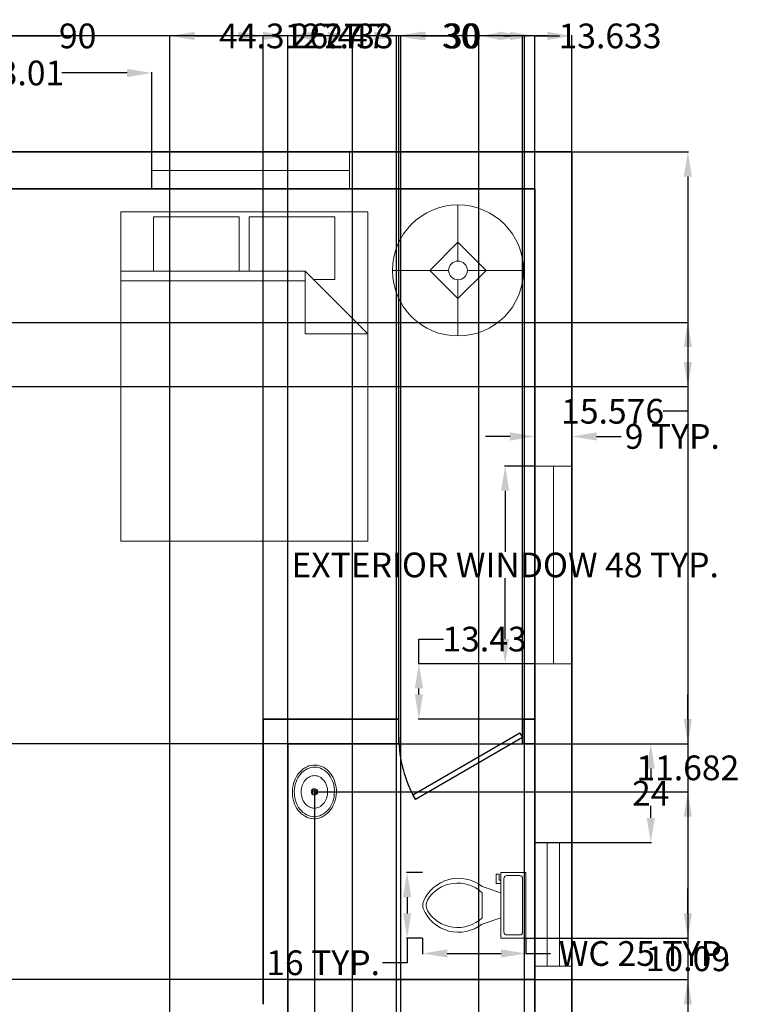
# Model space of a CAD drawing. Units: inches. Extents: x 351 to 774, y 111 to 703.
# Tile 6 of 6: x 599 to 774, y 464 to 703. Entities that reach past the tile are written whole.
import ezdxf

# ---------------------------------------------------------------- set-up
doc = ezdxf.new("R2010")
doc.units = ezdxf.units.IN
doc.header["$MEASUREMENT"] = 0
for name, color, linetype, lineweight in [('A-ANNO-DIMS', 2, 'Continuous', 18), ('A-DOOR', 3, 'Continuous', 25), ('A-FLOR-FIXT', 9, 'Continuous', 18), ('A-FURN', 8, 'Continuous', 18), ('A-GLAZ', 4, 'Continuous', 18), ('A-WALL', 7, 'Continuous', 35)]:
    doc.layers.add(name, color=color, linetype=linetype, lineweight=lineweight)
doc.styles.get("Standard").update_dxf_attribs({"font": 'arial.ttf'})
doc.dimstyles.get("Standard").update_dxf_attribs({"dimtxt": 6, "dimasz": 6, "dimexe": 0.18, "dimexo": 0.0625, "dimgap": 0.09, "dimtad": 0, "dimtih": 1, "dimtoh": 1, "dimdec": 0, "dimzin": 0, "dimdsep": 46, "dimlunit": 3, "dimtxsty": 'Standard', "dimcen": 0.09, "dimadec": 0, "dimazin": 0, "dimtfac": 1, "dimtdec": 0, "dimtofl": 0, "dimtmove": 0, "dimatfit": 3, "dimfxl": 1, "dimtolj": 1, "dimtzin": 0, "dimarcsym": 0})

# ---------------------------------------------------------------- blocks, each defined once
blk = doc.blocks.new('*U4')
for p, q in [((-40, 0), (-40, 6)), ((0, 0), (0, 6))]:
    blk.add_line(p, q)
blk.add_lwpolyline([(0, 0), (-34.64, -20), (-35.52, -18.48), (-0.88, 1.52)], close=True)
blk.add_arc((0, 0), 40, 180, 210)
blk = doc.blocks.new('Bed - Queen')
for p, q in [((0, -80.00003), (0, 0)), ((0, 0), (59.99999, 0)), ((59.99999, 0), (59.99999, -80.00003)), ((7.99999, -1.2), (28.79998, -1.2)), ((7.99999, -14.4), (7.99999, -1.2)), ((28.79998, -1.2), (28.79998, -14.4)), ((31.19999, -1.2), (51.99999, -1.2)), ((31.19999, -14.4), (31.19999, -1.2)), ((51.99999, -1.2), (51.99999, -16.4)), ((0, -14.4), (44.8, -14.4)), ((59.99999, -29.6), (44.8, -14.4)), ((44.8, -14.4), (44.8, -29.6)), ((51.99999, -16.4), (46.79936, -16.4)), ((44.8, -16.8), (0, -16.8)), ((44.8, -29.6), (59.99999, -29.6)), ((59.99999, -80.00003), (0, -80.00003))]:
    blk.add_line(p, q)
blk = doc.blocks.new('Lamp - Table')
for p, q in [((0, 7), (0, 1)), ((0, 3), (-3, 0)), ((3, 0), (0, 3)), ((-1, 0), (-7, 0)), ((-3, 0), (0, -3)), ((0, -3), (3, 0)), ((1, 0), (7, 0)), ((0, -1), (0, -7))]:
    blk.add_line(p, q)
for radius in [7, 1]:
    blk.add_circle((0, 0), radius)
blk = doc.blocks.new('Toilet - top')
for p, q in [((9.5, -6), (9.5, -2)), ((-10, -8.5), (-8, -8.5)), ((-10, -9.5), (-10, -8.5)), ((-8, -8.5), (-8, -8)), ((-7, -8), (-7, -9.5)), ((-4, -8), (-6, -14)), ((4, -8), (6, -14)), ((-7, -9.5), (-10, -9.5)), ((4, -14), (-4, -14))]:
    blk.add_line(p, q)
blk.add_lwpolyline([(10.5, -8), (10.5, 0), (-10.5, 0), (-10.5, -8)], close=True)
for points in [[(-9.5, -2), (-9.5, -6)], [(8.5, -1), (-8.5, -1)], [(-8.5, -7), (8.5, -7)]]:
    blk.add_lwpolyline(points)
for centre, radius, start, end in [((-8.62, -1.88), 0.884, 81.8699, 188.1301), ((8.62, -1.88), 0.884, 351.8699, 98.1301), ((-8.62, -6.12), 0.884, 171.8699, 278.1301), ((8.62, -6.12), 0.884, 261.8699, 8.1301), ((3.52, -21.58), 12.17, 141.4691, 247.9714), ((4.2, -21.82), 11.33, 136.3677, 238.9468), ((-3.52, -21.58), 12.17, 292.0284, 38.5307), ((-4.2, -21.82), 11.33, 301.053, 43.6321), ((0, -27.88), 4, 245.7318, 294.2682), ((0, -29), 4, 254.8605, 285.1395)]:
    blk.add_arc(centre, radius, start, end)
blk = doc.blocks.new('Sink - Oval top')
for p, q in [((-1, 0), (1, 0)), ((0, 1), (0, -1))]:
    blk.add_line(p, q)
for points in [[(-12.23, 0.39, 0.117634), (-11.46, -3.36, 0.104469), (-8.88, -6.8, 0.090016), (-5.08, -9.07, 0.08192), (-0.32, -10.02, 0.08192), (4.49, -9.38, 0.090016), (8.42, -7.36, 0.104469), (11.22, -4.09, 0.117634), (12.23, -0.39, 0.117634), (11.46, 3.36, 0.104469), (8.88, 6.8, 0.090016), (5.08, 9.07, 0.08192), (0.32, 10.02, 0.08192), (-4.49, 9.38, 0.090016), (-8.42, 7.36, 0.104469), (-11.22, 4.09, 0.117634)], [(-11.29, 0.16, 0.118622), (-10.52, -3.25, 0.104678), (-8.07, -6.36, 0.089562), (-4.54, -8.37, 0.081185), (-0.13, -9.15, 0.081185), (4.3, -8.49, 0.089562), (7.89, -6.58, 0.104678), (10.42, -3.55, 0.118622), (11.29, -0.16, 0.118622), (10.52, 3.25, 0.104678), (8.07, 6.36, 0.089562), (4.54, 8.37, 0.081185), (0.13, 9.15, 0.081185), (-4.3, 8.49, 0.089562), (-7.89, 6.58, 0.104678), (-10.42, 3.55, 0.118622)], [(-7.42, 0.08, 0.118283), (-6.91, -2.17, 0.104607), (-5.29, -4.21, 0.089718), (-2.97, -5.53, 0.081436), (-0.07, -6.04, 0.081436), (2.84, -5.59, 0.089718), (5.2, -4.33, 0.104607), (6.86, -2.32, 0.118283), (7.42, -0.08, 0.118283), (6.91, 2.17, 0.104607), (5.29, 4.21, 0.089718), (2.97, 5.53, 0.081436), (0.07, 6.04, 0.081436), (-2.84, 5.59, 0.089718), (-5.2, 4.33, 0.104607), (-6.86, 2.32, 0.118283)]]:
    blk.add_lwpolyline(points, format="xyb", close=True)
for radius in [1.5, 1]:
    blk.add_circle((0, 0), radius)
blk = doc.blocks.new('WIN-48IN-9IN-WALL')
blk.add_line((4.5, 48), (4.5, 0))
blk.add_lwpolyline([(0, 0), (9, 0), (9, 48), (0, 48)], close=True)
blk = doc.blocks.new('WIN-BATH-30IN-9IN-WALL')
for p, q in [((0, 0), (0, 9)), ((0, 9), (30, 9)), ((30, 9), (30, 0)), ((0, 6), (30, 6)), ((30, 3), (0, 3)), ((30, 0), (0, 0))]:
    blk.add_line(p, q)
blk = doc.blocks.new('*D24')
at = {"layer": 'A-ANNO-DIMS', "color": 0, "lineweight": -2, "transparency": 16777216}
for p, q in [((723.98, 594.93), (716.66, 594.93)), ((716.84, 588.93), (716.84, 574.13)), ((716.84, 552.93), (716.84, 567.74)), ((723.98, 546.93), (716.66, 546.93))]:
    blk.add_line(p, q, dxfattribs=at)
at = {"layer": 'A-ANNO-DIMS', "color": 0, "transparency": 16777216}
for points in [[(715.84, 588.93), (717.84, 588.93), (716.84, 594.93)], [(715.84, 552.93), (717.84, 552.93), (716.84, 546.93)]]:
    blk.add_solid(points, dxfattribs=at)
at = {"layer": 'Defpoints', "color": 0, "transparency": 16777216}
for p in [(716.84, 594.93), (724.04, 594.93), (724.04, 546.93)]:
    blk.add_point(p, dxfattribs=at)
at = {"layer": 'A-ANNO-DIMS', "color": 0, "transparency": 16777216, "insert": (716.84, 570.93), "char_height": 6, "attachment_point": 5}
blk.add_mtext('\\A1;EXTERIOR WINDOW 48 TYP.', dxfattribs=at)
blk = doc.blocks.new('*D25')
at = {"layer": 'A-ANNO-DIMS', "color": 0, "lineweight": -2, "transparency": 16777216}
for p, q in [((718.04, 602.13), (712.04, 602.13)), ((724.04, 594.99), (724.04, 602.31)), ((733.04, 594.99), (733.04, 602.31)), ((739.04, 602.13), (745.04, 602.13))]:
    blk.add_line(p, q, dxfattribs=at)
at = {"layer": 'A-ANNO-DIMS', "color": 0, "transparency": 16777216}
for points in [[(718.04, 603.13), (718.04, 601.13), (724.04, 602.13)], [(739.04, 603.13), (739.04, 601.13), (733.04, 602.13)]]:
    blk.add_solid(points, dxfattribs=at)
at = {"layer": 'Defpoints', "color": 0, "transparency": 16777216}
for p in [(733.04, 602.13), (724.04, 594.93), (733.04, 594.93)]:
    blk.add_point(p, dxfattribs=at)
at = {"layer": 'A-ANNO-DIMS', "color": 0, "transparency": 16777216, "insert": (757.41, 602.13), "char_height": 6, "attachment_point": 5}
blk.add_mtext('\\A1;9 TYP.', dxfattribs=at)
blk = doc.blocks.new('*D32')
at = {"layer": 'A-ANNO-DIMS', "color": 0, "lineweight": -2, "transparency": 16777216}
for p, q in [((696.79, 480.27), (696.79, 476.4)), ((721.84, 480.27), (721.84, 476.4)), ((702.79, 476.58), (715.84, 476.58)), ((721.84, 476.58), (727.84, 476.58))]:
    blk.add_line(p, q, dxfattribs=at)
at = {"layer": 'A-ANNO-DIMS', "color": 0, "transparency": 16777216}
for points in [[(702.79, 477.58), (702.79, 475.58), (696.79, 476.58)], [(715.84, 477.58), (715.84, 475.58), (721.84, 476.58)]]:
    blk.add_solid(points, dxfattribs=at)
at = {"layer": 'Defpoints', "color": 0, "transparency": 16777216}
for p in [(696.79, 480.33), (721.84, 480.33), (721.84, 476.58)]:
    blk.add_point(p, dxfattribs=at)
at = {"layer": 'A-ANNO-DIMS', "color": 0, "transparency": 16777216, "insert": (750.8, 476.58), "char_height": 6, "attachment_point": 5}
blk.add_mtext('\\A1;WC 25 TYP.', dxfattribs=at)
blk = doc.blocks.new('*D33')
at = {"layer": 'A-ANNO-DIMS', "color": 0, "lineweight": -2, "transparency": 16777216}
for p, q in [((696.73, 496.24), (692.86, 496.24)), ((693.04, 490.24), (693.04, 486.33)), ((696.73, 480.33), (692.86, 480.33)), ((693.04, 480.33), (693.04, 474.33)), ((693.04, 474.33), (687.04, 474.33))]:
    blk.add_line(p, q, dxfattribs=at)
at = {"layer": 'A-ANNO-DIMS', "color": 0, "transparency": 16777216}
for points in [[(692.04, 490.24), (694.04, 490.24), (693.04, 496.24)], [(692.04, 486.33), (694.04, 486.33), (693.04, 480.33)]]:
    blk.add_solid(points, dxfattribs=at)
at = {"layer": 'Defpoints', "color": 0, "transparency": 16777216}
for p in [(696.79, 496.24), (693.04, 480.33), (696.79, 480.33)]:
    blk.add_point(p, dxfattribs=at)
at = {"layer": 'A-ANNO-DIMS', "color": 0, "transparency": 16777216, "insert": (672.63, 474.33), "char_height": 6, "attachment_point": 5}
blk.add_mtext('\\A1;16 TYP.', dxfattribs=at)
blk = doc.blocks.new('*D46')
at = {"layer": 'A-ANNO-DIMS', "color": 0, "lineweight": -2, "transparency": 16777216}
for p, q in [((421.04, 671.3), (421.04, 699.57)), ((427.04, 699.39), (570.36, 699.39)), ((727.04, 699.39), (583.73, 699.39)), ((733.04, 671.3), (733.04, 699.57))]:
    blk.add_line(p, q, dxfattribs=at)
at = {"layer": 'A-ANNO-DIMS', "color": 0, "transparency": 16777216}
for points in [[(427.04, 700.39), (427.04, 698.39), (421.04, 699.39)], [(727.04, 700.39), (727.04, 698.39), (733.04, 699.39)]]:
    blk.add_solid(points, dxfattribs=at)
at = {"layer": 'Defpoints', "color": 0, "transparency": 16777216}
for p in [(733.04, 699.39), (421.04, 671.24), (733.04, 671.24)]:
    blk.add_point(p, dxfattribs=at)
at = {"layer": 'A-ANNO-DIMS', "color": 0, "transparency": 16777216, "insert": (577.04, 699.39), "char_height": 6, "attachment_point": 5}
blk.add_mtext('\\A1;312', dxfattribs=at)
blk = doc.blocks.new('*D47')
at = {"layer": 'A-ANNO-DIMS', "color": 0, "lineweight": -2, "transparency": 16777216}
for p, q in [((733.11, 671.24), (761.37, 671.24)), ((761.19, 665.24), (761.19, 410.4)), ((761.19, 149.24), (761.19, 404.09)), ((733.11, 143.24), (761.37, 143.24))]:
    blk.add_line(p, q, dxfattribs=at)
at = {"layer": 'A-ANNO-DIMS', "color": 0, "transparency": 16777216}
for points in [[(760.19, 665.24), (762.19, 665.24), (761.19, 671.24)], [(760.19, 149.24), (762.19, 149.24), (761.19, 143.24)]]:
    blk.add_solid(points, dxfattribs=at)
at = {"layer": 'Defpoints', "color": 0, "transparency": 16777216}
for p in [(733.04, 671.24), (761.19, 671.24), (733.04, 143.24)]:
    blk.add_point(p, dxfattribs=at)
at = {"layer": 'A-ANNO-DIMS', "color": 0, "transparency": 16777216, "insert": (761.19, 407.24), "char_height": 6, "attachment_point": 5}
blk.add_mtext('\\A1;528', dxfattribs=at)
blk = doc.blocks.new('*D51')
at = {"layer": 'A-ANNO-DIMS', "color": 0, "lineweight": -2, "transparency": 16777216}
for p, q in [((568.04, 662.3), (568.04, 690.57)), ((574.04, 690.39), (589.9, 690.39)), ((625.05, 690.39), (609.2, 690.39)), ((631.05, 662.3), (631.05, 690.57))]:
    blk.add_line(p, q, dxfattribs=at)
at = {"layer": 'A-ANNO-DIMS', "color": 0, "transparency": 16777216}
for points in [[(574.04, 691.39), (574.04, 689.39), (568.04, 690.39)], [(625.05, 691.39), (625.05, 689.39), (631.05, 690.39)]]:
    blk.add_solid(points, dxfattribs=at)
at = {"layer": 'Defpoints', "color": 0, "transparency": 16777216}
for p in [(631.05, 690.39), (568.04, 662.24), (631.05, 662.24)]:
    blk.add_point(p, dxfattribs=at)
at = {"layer": 'A-ANNO-DIMS', "color": 0, "transparency": 16777216, "insert": (599.55, 690.39), "char_height": 6, "attachment_point": 5}
blk.add_mtext('\\A1;63.01', dxfattribs=at)
blk = doc.blocks.new('*D64')
at = {"layer": 'A-ANNO-DIMS', "color": 0, "lineweight": -2, "transparency": 16777216}
for p, q in [((663.98, 527.5), (392.71, 527.5)), ((392.89, 521.5), (392.89, 502.02)), ((392.89, 476.24), (392.89, 495.72)), ((663.98, 470.24), (392.71, 470.24))]:
    blk.add_line(p, q, dxfattribs=at)
at = {"layer": 'A-ANNO-DIMS', "color": 0, "transparency": 16777216}
for points in [[(391.89, 521.5), (393.89, 521.5), (392.89, 527.5)], [(391.89, 476.24), (393.89, 476.24), (392.89, 470.24)]]:
    blk.add_solid(points, dxfattribs=at)
at = {"layer": 'Defpoints', "color": 0, "transparency": 16777216}
for p in [(392.89, 527.5), (664.04, 527.5), (664.04, 470.24)]:
    blk.add_point(p, dxfattribs=at)
at = {"layer": 'A-ANNO-DIMS', "color": 0, "transparency": 16777216, "insert": (392.89, 498.87), "char_height": 6, "attachment_point": 5}
blk.add_mtext('\\A1;57.26', dxfattribs=at)
blk = doc.blocks.new('*D65')
at = {"layer": 'A-ANNO-DIMS', "color": 0, "lineweight": -2, "transparency": 16777216}
for p, q in [((724.11, 527.5), (752.37, 527.5)), ((752.19, 521.5), (752.19, 518.6)), ((752.19, 509.5), (752.19, 512.4)), ((724.11, 503.5), (752.37, 503.5))]:
    blk.add_line(p, q, dxfattribs=at)
at = {"layer": 'A-ANNO-DIMS', "color": 0, "transparency": 16777216}
for points in [[(751.19, 521.5), (753.19, 521.5), (752.19, 527.5)], [(751.19, 509.5), (753.19, 509.5), (752.19, 503.5)]]:
    blk.add_solid(points, dxfattribs=at)
at = {"layer": 'Defpoints', "color": 0, "transparency": 16777216}
for p in [(724.04, 527.5), (724.04, 503.5), (752.19, 503.5)]:
    blk.add_point(p, dxfattribs=at)
at = {"layer": 'A-ANNO-DIMS', "color": 0, "transparency": 16777216, "insert": (752.19, 515.5), "char_height": 6, "attachment_point": 5}
blk.add_mtext('\\A1;24', dxfattribs=at)
blk = doc.blocks.new('*D66')
at = {"layer": 'A-ANNO-DIMS', "color": 0, "lineweight": -2, "transparency": 16777216}
for p, q in [((695.89, 546.93), (695.89, 552.93)), ((695.89, 552.93), (701.89, 552.93)), ((723.98, 546.93), (695.71, 546.93)), ((695.89, 539.5), (695.89, 540.93)), ((723.98, 533.5), (695.71, 533.5))]:
    blk.add_line(p, q, dxfattribs=at)
at = {"layer": 'A-ANNO-DIMS', "color": 0, "transparency": 16777216}
for points in [[(694.89, 540.93), (696.89, 540.93), (695.89, 546.93)], [(694.89, 539.5), (696.89, 539.5), (695.89, 533.5)]]:
    blk.add_solid(points, dxfattribs=at)
at = {"layer": 'Defpoints', "color": 0, "transparency": 16777216}
for p in [(695.89, 546.93), (724.04, 546.93), (724.04, 533.5)]:
    blk.add_point(p, dxfattribs=at)
at = {"layer": 'A-ANNO-DIMS', "color": 0, "transparency": 16777216, "insert": (711.82, 552.93), "char_height": 6, "attachment_point": 5}
blk.add_mtext('\\A1;13.43', dxfattribs=at)
blk = doc.blocks.new('*D69')
at = {"layer": 'A-ANNO-DIMS', "color": 0, "lineweight": -2, "transparency": 16777216}
for p, q in [((724.04, 473.44), (724.04, 114.91)), ((664.04, 470.18), (664.04, 114.91)), ((670.04, 115.09), (689.65, 115.09)), ((718.04, 115.09), (698.44, 115.09))]:
    blk.add_line(p, q, dxfattribs=at)
at = {"layer": 'A-ANNO-DIMS', "color": 0, "transparency": 16777216}
for points in [[(670.04, 116.09), (670.04, 114.09), (664.04, 115.09)], [(718.04, 116.09), (718.04, 114.09), (724.04, 115.09)]]:
    blk.add_solid(points, dxfattribs=at)
at = {"layer": 'Defpoints', "color": 0, "transparency": 16777216}
for p in [(724.04, 473.5), (664.04, 470.24), (724.04, 115.09)]:
    blk.add_point(p, dxfattribs=at)
at = {"layer": 'A-ANNO-DIMS', "color": 0, "transparency": 16777216, "insert": (694.04, 115.09), "char_height": 6, "attachment_point": 5}
blk.add_mtext('\\A1;60', dxfattribs=at)
blk = doc.blocks.new('*D80')
at = {"layer": 'A-ANNO-DIMS', "color": 0, "lineweight": -2, "transparency": 16777216}
for p, q in [((568.04, 464.3), (568.04, 699.57)), ((574.04, 699.39), (608.67, 699.39)), ((652.04, 699.39), (617.42, 699.39)), ((658.04, 464.3), (658.04, 699.57))]:
    blk.add_line(p, q, dxfattribs=at)
at = {"layer": 'A-ANNO-DIMS', "color": 0, "transparency": 16777216}
for points in [[(574.04, 700.39), (574.04, 698.39), (568.04, 699.39)], [(652.04, 700.39), (652.04, 698.39), (658.04, 699.39)]]:
    blk.add_solid(points, dxfattribs=at)
at = {"layer": 'Defpoints', "color": 0, "transparency": 16777216}
for p in [(658.04, 699.39), (568.04, 464.24), (658.04, 464.24)]:
    blk.add_point(p, dxfattribs=at)
at = {"layer": 'A-ANNO-DIMS', "color": 0, "transparency": 16777216, "insert": (613.04, 699.39), "char_height": 6, "attachment_point": 5}
blk.add_mtext('\\A1;90', dxfattribs=at)
blk = doc.blocks.new('*D86')
at = {"layer": 'A-ANNO-DIMS', "color": 0, "lineweight": -2, "transparency": 16777216}
for p, q in [((710.41, 152.3), (710.41, 699.57)), ((716.41, 699.39), (718.04, 699.39)), ((724.04, 152.3), (724.04, 699.57)), ((724.04, 699.39), (730.04, 699.39))]:
    blk.add_line(p, q, dxfattribs=at)
at = {"layer": 'A-ANNO-DIMS', "color": 0, "transparency": 16777216}
for points in [[(716.41, 700.39), (716.41, 698.39), (710.41, 699.39)], [(718.04, 700.39), (718.04, 698.39), (724.04, 699.39)]]:
    blk.add_solid(points, dxfattribs=at)
at = {"layer": 'Defpoints', "color": 0, "transparency": 16777216}
for p in [(724.04, 699.39), (710.41, 152.24), (724.04, 152.24)]:
    blk.add_point(p, dxfattribs=at)
at = {"layer": 'A-ANNO-DIMS', "color": 0, "transparency": 16777216, "insert": (742.3, 699.39), "char_height": 6, "attachment_point": 5}
blk.add_mtext('\\A1;13.633', dxfattribs=at)
blk = doc.blocks.new('*D87')
at = {"layer": 'A-ANNO-DIMS', "color": 0, "lineweight": -2, "transparency": 16777216}
for p, q in [((691.51, 206.3), (691.51, 699.57)), ((697.51, 699.39), (702.14, 699.39)), ((715.51, 699.39), (710.89, 699.39)), ((721.51, 206.3), (721.51, 699.57))]:
    blk.add_line(p, q, dxfattribs=at)
at = {"layer": 'A-ANNO-DIMS', "color": 0, "transparency": 16777216}
for points in [[(697.51, 700.39), (697.51, 698.39), (691.51, 699.39)], [(715.51, 700.39), (715.51, 698.39), (721.51, 699.39)]]:
    blk.add_solid(points, dxfattribs=at)
at = {"layer": 'Defpoints', "color": 0, "transparency": 16777216}
for p in [(721.51, 699.39), (691.51, 206.24), (721.51, 206.24)]:
    blk.add_point(p, dxfattribs=at)
at = {"layer": 'A-ANNO-DIMS', "color": 0, "transparency": 16777216, "insert": (706.51, 699.39), "char_height": 6, "attachment_point": 5}
blk.add_mtext('\\A1;30', dxfattribs=at)
blk = doc.blocks.new('*D88')
at = {"layer": 'A-ANNO-DIMS', "color": 0, "lineweight": -2, "transparency": 16777216}
for p, q in [((658.043027, 699.392076), (652.043027, 699.392076)), ((664.043027, 200.304576), (664.043027, 699.572076)), ((691.510725, 200.304576), (691.510725, 699.572076)), ((697.510725, 699.392076), (703.510725, 699.392076))]:
    blk.add_line(p, q, dxfattribs=at)
at = {"layer": 'A-ANNO-DIMS', "color": 0, "transparency": 16777216}
for points in [[(658.043027, 700.392076), (658.043027, 698.392076), (664.043027, 699.392076)], [(697.510725, 700.392076), (697.510725, 698.392076), (691.510725, 699.392076)]]:
    blk.add_solid(points, dxfattribs=at)
at = {"layer": 'Defpoints', "color": 0, "transparency": 16777216}
for p in [(691.510725, 699.392076), (664.043027, 200.242076), (691.510725, 200.242076)]:
    blk.add_point(p, dxfattribs=at)
at = {"layer": 'A-ANNO-DIMS', "color": 0, "transparency": 16777216, "insert": (677.776876, 699.392076), "char_height": 6, "attachment_point": 5}
blk.add_mtext('\\A1;27.47', dxfattribs=at)
blk = doc.blocks.new('*D89')
at = {"layer": 'A-ANNO-DIMS', "color": 0, "lineweight": -2, "transparency": 16777216}
for p, q in [((691.04, 533.56), (691.04, 699.57)), ((697.04, 699.39), (701.67, 699.39)), ((715.04, 699.39), (710.42, 699.39)), ((721.04, 533.56), (721.04, 699.57))]:
    blk.add_line(p, q, dxfattribs=at)
at = {"layer": 'A-ANNO-DIMS', "color": 0, "transparency": 16777216}
for points in [[(697.04, 700.39), (697.04, 698.39), (691.04, 699.39)], [(715.04, 700.39), (715.04, 698.39), (721.04, 699.39)]]:
    blk.add_solid(points, dxfattribs=at)
at = {"layer": 'Defpoints', "color": 0, "transparency": 16777216}
for p in [(721.04, 699.39), (691.04, 533.5), (721.04, 533.5)]:
    blk.add_point(p, dxfattribs=at)
at = {"layer": 'A-ANNO-DIMS', "color": 0, "transparency": 16777216, "insert": (706.04, 699.39), "char_height": 6, "attachment_point": 5}
blk.add_mtext('\\A1;30', dxfattribs=at)
blk = doc.blocks.new('*D90')
at = {"layer": 'A-ANNO-DIMS', "color": 0, "lineweight": -2, "transparency": 16777216}
for p, q in [((664.04, 527.56), (664.04, 699.57)), ((670.04, 699.39), (673.1, 699.39)), ((685.04, 699.39), (681.98, 699.39)), ((691.04, 527.56), (691.04, 699.57))]:
    blk.add_line(p, q, dxfattribs=at)
at = {"layer": 'A-ANNO-DIMS', "color": 0, "transparency": 16777216}
for points in [[(670.04, 700.39), (670.04, 698.39), (664.04, 699.39)], [(685.04, 700.39), (685.04, 698.39), (691.04, 699.39)]]:
    blk.add_solid(points, dxfattribs=at)
at = {"layer": 'Defpoints', "color": 0, "transparency": 16777216}
for p in [(691.04, 699.39), (664.04, 527.5), (691.04, 527.5)]:
    blk.add_point(p, dxfattribs=at)
at = {"layer": 'A-ANNO-DIMS', "color": 0, "transparency": 16777216, "insert": (677.54, 699.39), "char_height": 6, "attachment_point": 5}
blk.add_mtext('\\A1;27', dxfattribs=at)
blk = doc.blocks.new('*D96')
at = {"layer": 'A-ANNO-DIMS', "color": 0, "lineweight": -2, "transparency": 16777216}
for p, q in [((635.45, 422.7), (635.45, 699.57)), ((641.45, 699.39), (647.85, 699.39)), ((673.77, 699.39), (667.36, 699.39)), ((679.77, 423.87), (679.77, 699.57))]:
    blk.add_line(p, q, dxfattribs=at)
at = {"layer": 'A-ANNO-DIMS', "color": 0, "transparency": 16777216}
for points in [[(641.45, 700.39), (641.45, 698.39), (635.45, 699.39)], [(673.77, 700.39), (673.77, 698.39), (679.77, 699.39)]]:
    blk.add_solid(points, dxfattribs=at)
at = {"layer": 'Defpoints', "color": 0, "transparency": 16777216}
for p in [(679.77, 699.39), (679.77, 423.81), (635.45, 422.64)]:
    blk.add_point(p, dxfattribs=at)
at = {"layer": 'A-ANNO-DIMS', "color": 0, "transparency": 16777216, "insert": (657.61, 699.39), "char_height": 6, "attachment_point": 5}
blk.add_mtext('\\A1;44.31', dxfattribs=at)
blk = doc.blocks.new('*D98')
at = {"layer": 'A-ANNO-DIMS', "color": 0, "lineweight": -2, "transparency": 16777216}
for p, q in [((482.58, 629.82), (761.37, 629.82)), ((761.19, 623.82), (761.19, 620.24)), ((490.11, 614.24), (761.37, 614.24)), ((761.19, 614.24), (761.19, 608.24)), ((761.19, 608.24), (755.19, 608.24))]:
    blk.add_line(p, q, dxfattribs=at)
at = {"layer": 'A-ANNO-DIMS', "color": 0, "transparency": 16777216}
for points in [[(760.19, 623.82), (762.19, 623.82), (761.19, 629.82)], [(760.19, 620.24), (762.19, 620.24), (761.19, 614.24)]]:
    blk.add_solid(points, dxfattribs=at)
at = {"layer": 'Defpoints', "color": 0, "transparency": 16777216}
for p in [(482.51, 629.82), (490.04, 614.24), (761.19, 614.24)]:
    blk.add_point(p, dxfattribs=at)
at = {"layer": 'A-ANNO-DIMS', "color": 0, "transparency": 16777216, "insert": (742.93, 608.24), "char_height": 6, "attachment_point": 5}
blk.add_mtext('\\A1;15.576', dxfattribs=at)
blk = doc.blocks.new('*D101')
at = {"layer": 'A-ANNO-DIMS', "color": 0, "lineweight": -2, "transparency": 16777216}
for p, q in [((658.04, 699.39), (652.04, 699.39)), ((664.04, 152.3), (664.04, 699.57)), ((690.48, 153.55), (690.48, 699.57)), ((696.48, 699.39), (702.48, 699.39))]:
    blk.add_line(p, q, dxfattribs=at)
at = {"layer": 'A-ANNO-DIMS', "color": 0, "transparency": 16777216}
for points in [[(658.04, 700.39), (658.04, 698.39), (664.04, 699.39)], [(696.48, 700.39), (696.48, 698.39), (690.48, 699.39)]]:
    blk.add_solid(points, dxfattribs=at)
at = {"layer": 'Defpoints', "color": 0, "transparency": 16777216}
for p in [(664.04, 699.39), (690.48, 153.49), (664.04, 152.24)]:
    blk.add_point(p, dxfattribs=at)
at = {"layer": 'A-ANNO-DIMS', "color": 0, "transparency": 16777216, "insert": (677.26, 699.39), "char_height": 6, "attachment_point": 5}
blk.add_mtext('\\A1;26.433', dxfattribs=at)
blk = doc.blocks.new('*D103')
at = {"layer": 'A-ANNO-DIMS', "color": 0, "lineweight": -2, "transparency": 16777216}
for p, q in [((761.19, 486.33), (761.19, 492.33)), ((721.9, 480.33), (761.37, 480.33)), ((724.11, 470.24), (761.37, 470.24)), ((761.19, 464.24), (761.19, 458.24))]:
    blk.add_line(p, q, dxfattribs=at)
at = {"layer": 'A-ANNO-DIMS', "color": 0, "transparency": 16777216}
for points in [[(760.19, 486.33), (762.19, 486.33), (761.19, 480.33)], [(760.19, 464.24), (762.19, 464.24), (761.19, 470.24)]]:
    blk.add_solid(points, dxfattribs=at)
at = {"layer": 'Defpoints', "color": 0, "transparency": 16777216}
for p in [(721.84, 480.33), (724.04, 470.24), (761.19, 470.24)]:
    blk.add_point(p, dxfattribs=at)
at = {"layer": 'A-ANNO-DIMS', "color": 0, "transparency": 16777216, "insert": (761.19, 475.29), "char_height": 6, "attachment_point": 5}
blk.add_mtext('\\A1;10.09', dxfattribs=at)
blk = doc.blocks.new('*D104')
at = {"layer": 'A-ANNO-DIMS', "color": 0, "lineweight": -2, "transparency": 16777216}
for p, q in [((761.19, 533.5), (761.19, 539.5)), ((691.11, 527.5), (761.37, 527.5)), ((670.58, 515.82), (761.37, 515.82)), ((761.19, 509.82), (761.19, 503.82))]:
    blk.add_line(p, q, dxfattribs=at)
at = {"layer": 'A-ANNO-DIMS', "color": 0, "transparency": 16777216}
for points in [[(760.19, 533.5), (762.19, 533.5), (761.19, 527.5)], [(760.19, 509.82), (762.19, 509.82), (761.19, 515.82)]]:
    blk.add_solid(points, dxfattribs=at)
at = {"layer": 'Defpoints', "color": 0, "transparency": 16777216}
for p in [(691.04, 527.5), (761.19, 527.5), (670.51, 515.82)]:
    blk.add_point(p, dxfattribs=at)
at = {"layer": 'A-ANNO-DIMS', "color": 0, "transparency": 16777216, "insert": (761.19, 521.66), "char_height": 6, "attachment_point": 5}
blk.add_mtext('\\A1;11.682', dxfattribs=at)
blk = doc.blocks.new('*D108')
at = {"layer": 'A-ANNO-DIMS', "color": 0, "lineweight": -2, "transparency": 16777216}
for p, q in [((664.04, 527.44), (664.04, 114.91)), ((670.51, 515.76), (670.51, 114.91)), ((658.04, 115.09), (652.04, 115.09)), ((676.51, 115.09), (682.51, 115.09))]:
    blk.add_line(p, q, dxfattribs=at)
at = {"layer": 'A-ANNO-DIMS', "color": 0, "transparency": 16777216}
for points in [[(658.04, 116.09), (658.04, 114.09), (664.04, 115.09)], [(676.51, 116.09), (676.51, 114.09), (670.51, 115.09)]]:
    blk.add_solid(points, dxfattribs=at)
at = {"layer": 'Defpoints', "color": 0, "transparency": 16777216}
for p in [(664.04, 527.5), (670.51, 515.82), (664.04, 115.09)]:
    blk.add_point(p, dxfattribs=at)
at = {"layer": 'A-ANNO-DIMS', "color": 0, "transparency": 16777216, "insert": (641.84, 115.09), "char_height": 6, "attachment_point": 5}
blk.add_mtext('\\A1;6.472', dxfattribs=at)

msp = doc.modelspace()

# ---------------------------------------------------------------- linework, layer by layer
at = {"layer": 'A-WALL'}
for p, q in [((430.043, 662.2421), (724.043, 662.2421)), ((724.043, 662.2421), (724.043, 470.2421)), ((658.043, 533.5), (691.043, 533.5)), ((658.043, 533.5), (658.043, 515.2421)), ((721.043, 533.5), (724.043, 533.5)), ((664.043, 527.5), (691.043, 527.5)), ((664.043, 527.5), (664.043, 509.2421)), ((721.043, 527.5), (724.043, 527.5)), ((658.043, 515.2421), (658.043, 470.2421)), ((664.043, 509.2421), (664.043, 470.2421)), ((658.043, 470.2421), (658.043, 464.2421)), ((664.043, 470.2421), (724.043, 470.2421))]:
    msp.add_line(p, q, dxfattribs=at)
for points in [[(436.7781, 143.2421), (421.043, 143.2421), (421.043, 671.2421), (733.043, 671.2421), (733.043, 143.2421), (562.043, 143.2421)], [(721.043, 527.5), (721.043, 533.5)]]:
    msp.add_lwpolyline(points, dxfattribs=at)

# ---------------------------------------------------------------- block references
at = {"layer": 'A-DOOR', "xscale": 0.75, "yscale": 0.75, "zscale": 0.75}
msp.add_blockref('*U4', (721.043, 529), dxfattribs=at)
at = {"layer": 'A-FLOR-FIXT', "rotation": 270}
for name, p, xscale, yscale, zscale in [('Sink - Oval top', (670.5147, 515.8184), 0.53295403104476, 0.53295403104476, 0.53295403104476), ('Toilet - top', (721.8351, 488.2887), 0.7577391478424742, 0.7577391478424742, 0.7577391478424742)]:
    msp.add_blockref(name, p, dxfattribs=dict(at, xscale=xscale, yscale=yscale, zscale=zscale))
at = {"layer": 'A-FURN', "xscale": 2.273403864676251, "yscale": 2.273403864676251, "zscale": 2.273403864676251}
msp.add_blockref('Lamp - Table', (705.3835, 642.4481), dxfattribs=at)
at = {"layer": 'A-FURN'}
msp.add_blockref('Bed - Queen', (623.4803, 656.6822), dxfattribs=at)
at = {"layer": 'A-GLAZ'}
for name, p, rotation in [('WIN-48IN-9IN-WALL', (679.0513, 662.2421), 90.00000000000003), ('WIN-BATH-30IN-9IN-WALL', (733.043, 473.5), 90.0000000000016)]:
    msp.add_blockref(name, p, dxfattribs=dict(at, rotation=rotation))
msp.add_blockref('WIN-48IN-9IN-WALL', (724.043, 546.9313), dxfattribs=at)

# ---------------------------------------------------------------- dimensions: what is measured, and where the dimension line sits
at = {"layer": 'A-ANNO-DIMS'}
for base, p1, p2, override, picture, middle in [((733.043, 699.3921), (421.043, 671.2421), (733.043, 671.2421), {"dimdec": 0, "dimlfac": 1, "dimrnd": 0, "dimzin": 0, "dimdsep": 46, "dimlunit": 2}, '*D46', (577.043, 699.3921)), ((658.043, 699.3921), (568.043, 464.2421), (658.043, 464.2421), {"dimdec": 0, "dimlfac": 1, "dimrnd": 0, "dimzin": 0, "dimdsep": 46, "dimlunit": 2}, '*D80', (613.043, 699.3921)), ((679.7664, 699.3921), (635.4531, 422.6419), (679.7664, 423.8083), {"dimdec": 2, "dimlfac": 1, "dimrnd": 0, "dimzin": 0, "dimdsep": 46, "dimlunit": 2}, '*D96', (657.6098, 699.3921)), ((691.5107, 699.3921), (664.043, 200.2421), (691.5107, 200.2421), {"dimdec": 2, "dimlfac": 1, "dimrnd": 0, "dimzin": 0, "dimdsep": 46, "dimlunit": 2}, '*D88', (677.7769, 699.3921)), ((664.043, 699.3921), (690.4757, 153.4918), (664.043, 152.2421), {"dimdec": 3, "dimlfac": 1, "dimrnd": 0, "dimzin": 0, "dimdsep": 46, "dimlunit": 2}, '*D101', (677.2594, 699.3921)), ((691.043, 699.3921), (664.043, 527.5), (691.043, 527.5), {"dimdec": 0, "dimlfac": 1, "dimrnd": 0, "dimzin": 0, "dimdsep": 46, "dimlunit": 2}, '*D90', (677.543, 699.3921)), ((721.043, 699.3921), (691.043, 533.5), (721.043, 533.5), {"dimdec": 0, "dimlfac": 1, "dimrnd": 0, "dimzin": 0, "dimdsep": 46, "dimlunit": 2}, '*D89', (706.043, 699.3921)), ((721.5107, 699.3921), (691.5107, 206.2421), (721.5107, 206.2421), {"dimdec": 0, "dimlfac": 1, "dimrnd": 0, "dimzin": 0, "dimdsep": 46, "dimlunit": 2}, '*D87', (706.5107, 699.3921)), ((724.043, 699.3921), (710.4102, 152.2421), (724.043, 152.2421), {"dimdec": 3, "dimlfac": 1, "dimrnd": 0, "dimzin": 0, "dimdsep": 46, "dimlunit": 2}, '*D86', (742.3049, 699.3921)), ((631.0513, 690.3921), (568.043, 662.2421), (631.0513, 662.2421), {"dimdec": 2, "dimlfac": 1, "dimrnd": 0, "dimzin": 0, "dimdsep": 46, "dimlunit": 2}, '*D51', (599.5471, 690.3921)), ((664.043, 115.0921), (670.5147, 515.8184), (664.043, 527.5), {"dimdec": 3, "dimlfac": 1, "dimrnd": 0, "dimzin": 0, "dimdsep": 46, "dimlunit": 2}, '*D108', (641.8439, 115.0921)), ((724.043, 115.0921), (664.043, 470.2421), (724.043, 473.5), {"dimdec": 0, "dimlfac": 1, "dimrnd": 0, "dimzin": 0, "dimdsep": 46, "dimlunit": 2}, '*D69', (694.043, 115.0921))]:
    dim = msp.add_linear_dim(base=base, p1=p1, p2=p2, dimstyle='Standard', override=override, dxfattribs=at)
    dim.commit()
    dim.dimension.update_dxf_attribs({"geometry": picture, "text_midpoint": middle})
for base, p1, p2, angle, override, picture, middle in [((761.193, 671.2421), (733.043, 143.2421), (733.043, 671.2421), 90, {"dimdec": 0, "dimlfac": 1, "dimrnd": 0, "dimzin": 0, "dimdsep": 46, "dimlunit": 2}, '*D47', (761.193, 407.2421)), ((761.193, 614.2421), (482.5147, 629.8184), (490.043, 614.2421), 90, {"dimdec": 3, "dimlfac": 1, "dimrnd": 0, "dimzin": 0, "dimdsep": 46, "dimlunit": 2}, '*D98', (742.9332, 608.2421)), ((695.893, 546.9313), (724.043, 533.5), (724.043, 546.9313), 90, {"dimdec": 2, "dimlfac": 1, "dimrnd": 0, "dimzin": 0, "dimdsep": 46, "dimlunit": 2}, '*D66', (711.8241, 552.9313)), ((761.193, 527.5), (670.5147, 515.8184), (691.043, 527.5), 90, {"dimdec": 3, "dimlfac": 1, "dimrnd": 0, "dimzin": 0, "dimdsep": 46, "dimlunit": 2}, '*D104', (761.193, 521.6592)), ((392.893, 527.5), (664.043, 470.2421), (664.043, 527.5), 90, {"dimdec": 2, "dimlfac": 1, "dimrnd": 0, "dimzin": 0, "dimdsep": 46, "dimlunit": 2}, '*D64', (392.893, 498.871)), ((752.193, 503.5), (724.043, 527.5), (724.043, 503.5), 270, {"dimdec": 0, "dimlfac": 1, "dimrnd": 0, "dimzin": 0, "dimdsep": 46, "dimlunit": 2}, '*D65', (752.193, 515.5)), ((761.193, 470.2421), (721.8351, 480.3324), (724.043, 470.2421), 90, {"dimdec": 2, "dimlfac": 1, "dimrnd": 0, "dimzin": 0, "dimdsep": 46, "dimlunit": 2}, '*D103', (761.193, 475.2873))]:
    dim = msp.add_linear_dim(base=base, p1=p1, p2=p2, angle=angle, dimstyle='Standard', override=override, dxfattribs=at)
    dim.commit()
    dim.dimension.update_dxf_attribs({"geometry": picture, "text_midpoint": middle})
for base, p1, p2, text, picture, middle in [((733.043, 602.1313), (724.043, 594.9313), (733.043, 594.9313), '<> TYP.', '*D25', (757.4052, 602.1313)), ((721.8351, 476.5764), (696.7947, 480.3324), (721.8351, 480.3324), 'WC <> TYP.', '*D32', (750.7976, 476.5764))]:
    dim = msp.add_linear_dim(base=base, p1=p1, p2=p2, text=text, dimstyle='Standard', override={"dimdec": 0, "dimlfac": 1, "dimrnd": 0, "dimzin": 0, "dimdsep": 46, "dimlunit": 2}, dxfattribs=at)
    dim.commit()
    dim.dimension.update_dxf_attribs({"geometry": picture, "text_midpoint": middle})
for base, p1, p2, angle, text, picture, middle in [((716.843, 594.9313), (724.043, 546.9313), (724.043, 594.9313), 90, 'EXTERIOR WINDOW <> TYP.', '*D24', (716.843, 570.9313)), ((693.0386, 480.3324), (696.7947, 496.245), (696.7947, 480.3324), 270, '<> TYP.', '*D33', (672.628, 474.3324))]:
    dim = msp.add_linear_dim(base=base, p1=p1, p2=p2, angle=angle, text=text, dimstyle='Standard', override={"dimdec": 0, "dimlfac": 1, "dimrnd": 0, "dimzin": 0, "dimdsep": 46, "dimlunit": 2}, dxfattribs=at)
    dim.commit()
    dim.dimension.update_dxf_attribs({"geometry": picture, "text_midpoint": middle})

doc.saveas('drawing.dxf')
